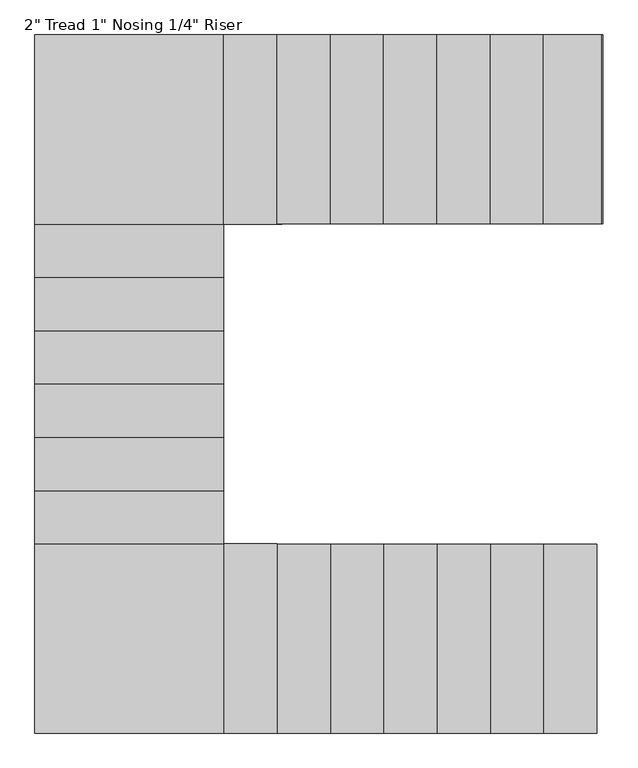
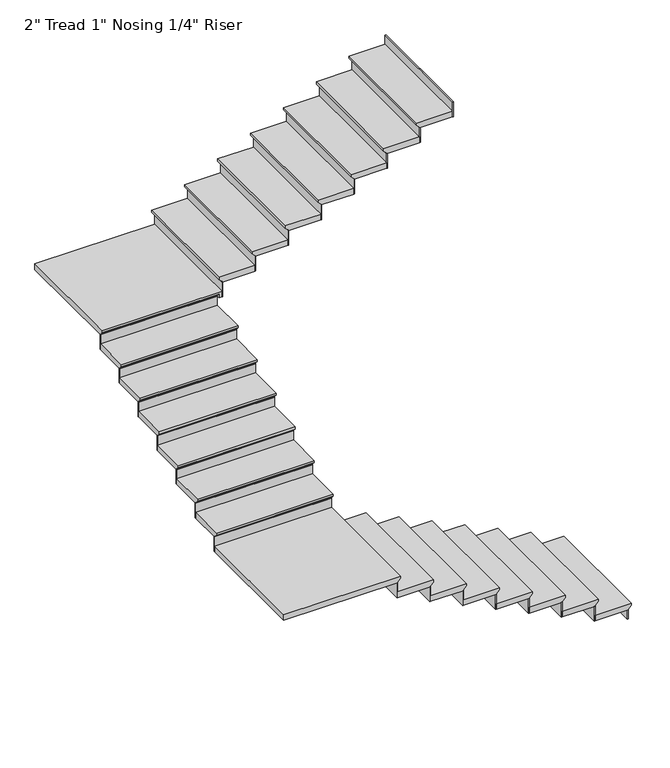
"""IFC4 building model written with IfcOpenShell, lengths in millimetres: stair flight geometry."""

from ifc_helpers import new_model, si_unit, origin, place, context, project, spatial, faceted_brep, source, transform, mapped, element, save


def stair_flight_9d362d5c(model_context):
    return source(origin(), model_context, "Body", "Brep", [
        faceted_brep([(-19769.8789184, -127.8399287, 3161.4717391), (-19769.8789184, -127.8399287, 3180.5217391), (-19769.8789184, -1118.4399287, 3180.5217391), (-19769.8789184, -1118.4399287, 3161.4717391), (-19795.2789184, -127.8399287, 3136.0717391), (-19795.2789184, -1118.4399287, 3136.0717391), (-20074.6789184, -127.8399287, 3180.5217391), (-20074.6789184, -1118.4399287, 3180.5217391), (-19795.2789184, -1118.4399287, 3129.7217391), (-20074.6789184, -1118.4399287, 3129.7217391), (-20074.6789184, -127.8399287, 3129.7217391), (-19795.2789184, -127.8399287, 3129.7217391)], [[[0, 1, 2, 3]], [[4, 0, 3, 5]], [[2, 1, 6, 7]], [[8, 9, 10, 11]], [[2, 7, 9, 8, 5, 3]], [[8, 11, 4, 5]], [[6, 1, 0, 4, 11, 10]], [[7, 6, 10, 9]]]),
        faceted_brep([(-19795.2789184, -127.8399287, 3129.7217391), (-19795.2789184, -127.8399287, 3048.0), (-19801.6289184, -127.8399287, 3048.0), (-19801.6289184, -127.8399287, 3129.7217391), (-19795.2789184, -1118.4399287, 3129.7217391), (-19801.6289184, -1118.4399287, 3129.7217391), (-19801.6289184, -1118.4399287, 3048.0), (-19795.2789184, -1118.4399287, 3048.0)], [[[0, 1, 2, 3]], [[4, 5, 6, 7]], [[1, 0, 4, 7]], [[2, 1, 7, 6]], [[3, 2, 6, 5]], [[0, 3, 5, 4]]]),
        faceted_brep([(-20074.6789184, -127.8399287, 3262.2434783), (-20074.6789184, -127.8399287, 3129.7217391), (-20081.0289184, -127.8399287, 3129.7217391), (-20081.0289184, -127.8399287, 3262.2434783), (-20074.6789184, -1118.4399287, 3262.2434783), (-20081.0289184, -1118.4399287, 3262.2434783), (-20081.0289184, -1118.4399287, 3129.7217391), (-20074.6789184, -1118.4399287, 3129.7217391)], [[[0, 1, 2, 3]], [[4, 5, 6, 7]], [[1, 0, 4, 7]], [[2, 1, 7, 6]], [[3, 2, 6, 5]], [[0, 3, 5, 4]]]),
        faceted_brep([(-20049.2789184, -1118.4399287, 3313.0434783), (-20049.2789184, -127.8399287, 3313.0434783), (-20354.0789184, -127.8399287, 3313.0434783), (-20354.0789184, -1118.4399287, 3313.0434783), (-20074.6789184, -1118.4399287, 3262.2434783), (-20354.0789184, -1118.4399287, 3262.2434783), (-20354.0789184, -127.8399287, 3262.2434783), (-20074.6789184, -127.8399287, 3262.2434783), (-20074.6789184, -1118.4399287, 3268.5934783), (-20049.2789184, -1118.4399287, 3293.9934783), (-20074.6789184, -127.8399287, 3268.5934783), (-20049.2789184, -127.8399287, 3293.9934783)], [[[0, 1, 2, 3]], [[4, 5, 6, 7]], [[0, 3, 5, 4, 8, 9]], [[4, 7, 10, 8]], [[2, 1, 11, 10, 7, 6]], [[3, 2, 6, 5]], [[11, 1, 0, 9]], [[10, 11, 9, 8]]]),
        faceted_brep([(-20354.0789184, -127.8399287, 3394.7652174), (-20354.0789184, -127.8399287, 3262.2434783), (-20360.4289184, -127.8399287, 3262.2434783), (-20360.4289184, -127.8399287, 3394.7652174), (-20354.0789184, -1118.4399287, 3394.7652174), (-20360.4289184, -1118.4399287, 3394.7652174), (-20360.4289184, -1118.4399287, 3262.2434783), (-20354.0789184, -1118.4399287, 3262.2434783)], [[[0, 1, 2, 3]], [[4, 5, 6, 7]], [[1, 0, 4, 7]], [[2, 1, 7, 6]], [[3, 2, 6, 5]], [[0, 3, 5, 4]]]),
        faceted_brep([(-20328.6789184, -1118.4399287, 3445.5652174), (-20328.6789184, -127.8399287, 3445.5652174), (-20633.4789184, -127.8399287, 3445.5652174), (-20633.4789184, -1118.4399287, 3445.5652174), (-20354.0789184, -1118.4399287, 3394.7652174), (-20633.4789184, -1118.4399287, 3394.7652174), (-20633.4789184, -127.8399287, 3394.7652174), (-20354.0789184, -127.8399287, 3394.7652174), (-20354.0789184, -1118.4399287, 3401.1152174), (-20328.6789184, -1118.4399287, 3426.5152174), (-20354.0789184, -127.8399287, 3401.1152174), (-20328.6789184, -127.8399287, 3426.5152174)], [[[0, 1, 2, 3]], [[4, 5, 6, 7]], [[0, 3, 5, 4, 8, 9]], [[4, 7, 10, 8]], [[2, 1, 11, 10, 7, 6]], [[3, 2, 6, 5]], [[11, 1, 0, 9]], [[10, 11, 9, 8]]]),
        faceted_brep([(-20633.4789184, -127.8399287, 3527.2869565), (-20633.4789184, -127.8399287, 3394.7652174), (-20639.8289184, -127.8399287, 3394.7652174), (-20639.8289184, -127.8399287, 3527.2869565), (-20633.4789184, -1118.4399287, 3527.2869565), (-20639.8289184, -1118.4399287, 3527.2869565), (-20639.8289184, -1118.4399287, 3394.7652174), (-20633.4789184, -1118.4399287, 3394.7652174)], [[[0, 1, 2, 3]], [[4, 5, 6, 7]], [[1, 0, 4, 7]], [[2, 1, 7, 6]], [[3, 2, 6, 5]], [[0, 3, 5, 4]]]),
        faceted_brep([(-20608.0789184, -1118.4399287, 3578.0869565), (-20608.0789184, -127.8399287, 3578.0869565), (-20912.8789184, -127.8399287, 3578.0869565), (-20912.8789184, -1118.4399287, 3578.0869565), (-20633.4789184, -1118.4399287, 3527.2869565), (-20912.8789184, -1118.4399287, 3527.2869565), (-20912.8789184, -127.8399287, 3527.2869565), (-20633.4789184, -127.8399287, 3527.2869565), (-20633.4789184, -1118.4399287, 3533.6369565), (-20608.0789184, -1118.4399287, 3559.0369565), (-20633.4789184, -127.8399287, 3533.6369565), (-20608.0789184, -127.8399287, 3559.0369565)], [[[0, 1, 2, 3]], [[4, 5, 6, 7]], [[0, 3, 5, 4, 8, 9]], [[4, 7, 10, 8]], [[2, 1, 11, 10, 7, 6]], [[3, 2, 6, 5]], [[11, 1, 0, 9]], [[10, 11, 9, 8]]]),
        faceted_brep([(-20912.8789184, -127.8399287, 3659.8086957), (-20912.8789184, -127.8399287, 3527.2869565), (-20919.2289184, -127.8399287, 3527.2869565), (-20919.2289184, -127.8399287, 3659.8086957), (-20912.8789184, -1118.4399287, 3659.8086957), (-20919.2289184, -1118.4399287, 3659.8086957), (-20919.2289184, -1118.4399287, 3527.2869565), (-20912.8789184, -1118.4399287, 3527.2869565)], [[[0, 1, 2, 3]], [[4, 5, 6, 7]], [[1, 0, 4, 7]], [[2, 1, 7, 6]], [[3, 2, 6, 5]], [[0, 3, 5, 4]]]),
        faceted_brep([(-20887.4789184, -1118.4399287, 3710.6086957), (-20887.4789184, -127.8399287, 3710.6086957), (-21192.2789184, -127.8399287, 3710.6086957), (-21192.2789184, -1118.4399287, 3710.6086957), (-20912.8789184, -1118.4399287, 3659.8086957), (-21192.2789184, -1118.4399287, 3659.8086957), (-21192.2789184, -127.8399287, 3659.8086957), (-20912.8789184, -127.8399287, 3659.8086957), (-20912.8789184, -1118.4399287, 3666.1586957), (-20887.4789184, -1118.4399287, 3691.5586957), (-20912.8789184, -127.8399287, 3666.1586957), (-20887.4789184, -127.8399287, 3691.5586957)], [[[0, 1, 2, 3]], [[4, 5, 6, 7]], [[0, 3, 5, 4, 8, 9]], [[4, 7, 10, 8]], [[2, 1, 11, 10, 7, 6]], [[3, 2, 6, 5]], [[11, 1, 0, 9]], [[10, 11, 9, 8]]]),
        faceted_brep([(-21192.2789184, -127.8399287, 3792.3304348), (-21192.2789184, -127.8399287, 3659.8086957), (-21198.6289184, -127.8399287, 3659.8086957), (-21198.6289184, -127.8399287, 3792.3304348), (-21192.2789184, -1118.4399287, 3792.3304348), (-21198.6289184, -1118.4399287, 3792.3304348), (-21198.6289184, -1118.4399287, 3659.8086957), (-21192.2789184, -1118.4399287, 3659.8086957)], [[[0, 1, 2, 3]], [[4, 5, 6, 7]], [[1, 0, 4, 7]], [[2, 1, 7, 6]], [[3, 2, 6, 5]], [[0, 3, 5, 4]]]),
        faceted_brep([(-21166.8789184, -1118.4399287, 3843.1304348), (-21166.8789184, -127.8399287, 3843.1304348), (-21471.6789184, -127.8399287, 3843.1304348), (-21471.6789184, -1118.4399287, 3843.1304348), (-21192.2789184, -1118.4399287, 3792.3304348), (-21471.6789184, -1118.4399287, 3792.3304348), (-21471.6789184, -127.8399287, 3792.3304348), (-21192.2789184, -127.8399287, 3792.3304348), (-21192.2789184, -1118.4399287, 3798.6804348), (-21166.8789184, -1118.4399287, 3824.0804348), (-21192.2789184, -127.8399287, 3798.6804348), (-21166.8789184, -127.8399287, 3824.0804348)], [[[0, 1, 2, 3]], [[4, 5, 6, 7]], [[0, 3, 5, 4, 8, 9]], [[4, 7, 10, 8]], [[2, 1, 11, 10, 7, 6]], [[3, 2, 6, 5]], [[11, 1, 0, 9]], [[10, 11, 9, 8]]]),
        faceted_brep([(-21471.6789184, -127.8399287, 3924.8521739), (-21471.6789184, -127.8399287, 3792.3304348), (-21478.0289184, -127.8399287, 3792.3304348), (-21478.0289184, -127.8399287, 3924.8521739), (-21471.6789184, -1118.4399287, 3924.8521739), (-21478.0289184, -1118.4399287, 3924.8521739), (-21478.0289184, -1118.4399287, 3792.3304348), (-21471.6789184, -1118.4399287, 3792.3304348)], [[[0, 1, 2, 3]], [[4, 5, 6, 7]], [[1, 0, 4, 7]], [[2, 1, 7, 6]], [[3, 2, 6, 5]], [[0, 3, 5, 4]]]),
        faceted_brep([(-21446.2789184, -1118.4399287, 3975.6521739), (-21446.2789184, -127.8399287, 3975.6521739), (-21751.0789184, -127.8399287, 3975.6521739), (-21751.0789184, -1118.4399287, 3975.6521739), (-21471.6789184, -1118.4399287, 3924.8521739), (-21751.0789184, -1118.4399287, 3924.8521739), (-21751.0789184, -127.8399287, 3924.8521739), (-21471.6789184, -127.8399287, 3924.8521739), (-21471.6789184, -1118.4399287, 3931.2021739), (-21446.2789184, -1118.4399287, 3956.6021739), (-21471.6789184, -127.8399287, 3931.2021739), (-21446.2789184, -127.8399287, 3956.6021739)], [[[0, 1, 2, 3]], [[4, 5, 6, 7]], [[0, 3, 5, 4, 8, 9]], [[4, 7, 10, 8]], [[2, 1, 11, 10, 7, 6]], [[3, 2, 6, 5]], [[11, 1, 0, 9]], [[10, 11, 9, 8]]]),
        faceted_brep([(-21751.0789184, -127.8399287, 4057.373913), (-21751.0789184, -127.8399287, 3924.8521739), (-21757.4289184, -127.8399287, 3924.8521739), (-21757.4289184, -127.8399287, 4057.373913), (-21751.0789184, -1118.4399287, 4057.373913), (-21757.4289184, -1118.4399287, 4057.373913), (-21757.4289184, -1118.4399287, 3924.8521739), (-21751.0789184, -1118.4399287, 3924.8521739)], [[[0, 1, 2, 3]], [[4, 5, 6, 7]], [[1, 0, 4, 7]], [[2, 1, 7, 6]], [[3, 2, 6, 5]], [[0, 3, 5, 4]]]),
        faceted_brep([(-22716.2789184, -102.4399287, 4108.173913), (-22716.2789184, -1118.4399287, 4108.173913), (-21725.6789184, -1118.4399287, 4108.173913), (-21725.6789184, -102.4399287, 4108.173913), (-22716.2789184, -1118.4399287, 4057.373913), (-22716.2789184, -102.4399287, 4057.373913), (-21725.6789184, -102.4399287, 4057.373913), (-21725.6789184, -127.8399287, 4057.373913), (-21751.0789184, -127.8399287, 4057.373913), (-21751.0789184, -1118.4399287, 4057.373913), (-21751.0789184, -127.8399287, 4063.723913), (-21751.0789184, -1118.4399287, 4063.723913), (-21725.6789184, -1118.4399287, 4089.123913), (-21725.6789184, -127.8399287, 4089.123913)], [[[0, 1, 2, 3]], [[4, 5, 6, 7, 8, 9]], [[1, 0, 5, 4]], [[9, 8, 10, 11]], [[3, 2, 12, 13, 7, 6]], [[0, 3, 6, 5]], [[12, 11, 10, 13]], [[2, 1, 4, 9, 11, 12]], [[8, 7, 13, 10]]]),
        faceted_brep([(-21725.6789184, -102.4399287, 4189.8956522), (-21725.6789184, -102.4399287, 4057.373913), (-21725.6789184, -96.0899287, 4057.373913), (-21725.6789184, -96.0899287, 4189.8956522), (-22716.2789184, -102.4399287, 4189.8956522), (-22716.2789184, -96.0899287, 4189.8956522), (-22716.2789184, -96.0899287, 4057.373913), (-22716.2789184, -102.4399287, 4057.373913)], [[[0, 1, 2, 3]], [[4, 5, 6, 7]], [[1, 0, 4, 7]], [[2, 1, 7, 6]], [[3, 2, 6, 5]], [[0, 3, 5, 4]]]),
        faceted_brep([(-22716.2789184, -127.8399287, 4240.6956522), (-21725.6789184, -127.8399287, 4240.6956522), (-21725.6789184, 176.9600713, 4240.6956522), (-22716.2789184, 176.9600713, 4240.6956522), (-22716.2789184, -102.4399287, 4189.8956522), (-22716.2789184, 176.9600713, 4189.8956522), (-21725.6789184, 176.9600713, 4189.8956522), (-21725.6789184, -102.4399287, 4189.8956522), (-22716.2789184, -102.4399287, 4196.2456522), (-22716.2789184, -127.8399287, 4221.6456522), (-21725.6789184, -102.4399287, 4196.2456522), (-21725.6789184, -127.8399287, 4221.6456522)], [[[0, 1, 2, 3]], [[4, 5, 6, 7]], [[0, 3, 5, 4, 8, 9]], [[4, 7, 10, 8]], [[2, 1, 11, 10, 7, 6]], [[3, 2, 6, 5]], [[11, 1, 0, 9]], [[10, 11, 9, 8]]]),
        faceted_brep([(-21725.6789184, 176.9600713, 4322.4173913), (-21725.6789184, 176.9600713, 4189.8956522), (-21725.6789184, 183.3100713, 4189.8956522), (-21725.6789184, 183.3100713, 4322.4173913), (-22716.2789184, 176.9600713, 4322.4173913), (-22716.2789184, 183.3100713, 4322.4173913), (-22716.2789184, 183.3100713, 4189.8956522), (-22716.2789184, 176.9600713, 4189.8956522)], [[[0, 1, 2, 3]], [[4, 5, 6, 7]], [[1, 0, 4, 7]], [[2, 1, 7, 6]], [[3, 2, 6, 5]], [[0, 3, 5, 4]]]),
        faceted_brep([(-22716.2789184, 151.5600713, 4373.2173913), (-21725.6789184, 151.5600713, 4373.2173913), (-21725.6789184, 456.3600713, 4373.2173913), (-22716.2789184, 456.3600713, 4373.2173913), (-22716.2789184, 176.9600713, 4322.4173913), (-22716.2789184, 456.3600713, 4322.4173913), (-21725.6789184, 456.3600713, 4322.4173913), (-21725.6789184, 176.9600713, 4322.4173913), (-22716.2789184, 176.9600713, 4328.7673913), (-22716.2789184, 151.5600713, 4354.1673913), (-21725.6789184, 176.9600713, 4328.7673913), (-21725.6789184, 151.5600713, 4354.1673913)], [[[0, 1, 2, 3]], [[4, 5, 6, 7]], [[0, 3, 5, 4, 8, 9]], [[4, 7, 10, 8]], [[2, 1, 11, 10, 7, 6]], [[3, 2, 6, 5]], [[11, 1, 0, 9]], [[10, 11, 9, 8]]]),
        faceted_brep([(-21725.6789184, 456.3600713, 4454.9391304), (-21725.6789184, 456.3600713, 4322.4173913), (-21725.6789184, 462.7100713, 4322.4173913), (-21725.6789184, 462.7100713, 4454.9391304), (-22716.2789184, 456.3600713, 4454.9391304), (-22716.2789184, 462.7100713, 4454.9391304), (-22716.2789184, 462.7100713, 4322.4173913), (-22716.2789184, 456.3600713, 4322.4173913)], [[[0, 1, 2, 3]], [[4, 5, 6, 7]], [[1, 0, 4, 7]], [[2, 1, 7, 6]], [[3, 2, 6, 5]], [[0, 3, 5, 4]]]),
        faceted_brep([(-22716.2789184, 430.9600713, 4505.7391304), (-21725.6789184, 430.9600713, 4505.7391304), (-21725.6789184, 735.7600713, 4505.7391304), (-22716.2789184, 735.7600713, 4505.7391304), (-22716.2789184, 456.3600713, 4454.9391304), (-22716.2789184, 735.7600713, 4454.9391304), (-21725.6789184, 735.7600713, 4454.9391304), (-21725.6789184, 456.3600713, 4454.9391304), (-22716.2789184, 456.3600713, 4461.2891304), (-22716.2789184, 430.9600713, 4486.6891304), (-21725.6789184, 456.3600713, 4461.2891304), (-21725.6789184, 430.9600713, 4486.6891304)], [[[0, 1, 2, 3]], [[4, 5, 6, 7]], [[0, 3, 5, 4, 8, 9]], [[4, 7, 10, 8]], [[2, 1, 11, 10, 7, 6]], [[3, 2, 6, 5]], [[11, 1, 0, 9]], [[10, 11, 9, 8]]]),
        faceted_brep([(-21725.6789184, 735.7600713, 4587.4608696), (-21725.6789184, 735.7600713, 4454.9391304), (-21725.6789184, 742.1100713, 4454.9391304), (-21725.6789184, 742.1100713, 4587.4608696), (-22716.2789184, 735.7600713, 4587.4608696), (-22716.2789184, 742.1100713, 4587.4608696), (-22716.2789184, 742.1100713, 4454.9391304), (-22716.2789184, 735.7600713, 4454.9391304)], [[[0, 1, 2, 3]], [[4, 5, 6, 7]], [[1, 0, 4, 7]], [[2, 1, 7, 6]], [[3, 2, 6, 5]], [[0, 3, 5, 4]]]),
        faceted_brep([(-22716.2789184, 710.3600713, 4638.2608696), (-21725.6789184, 710.3600713, 4638.2608696), (-21725.6789184, 1015.1600713, 4638.2608696), (-22716.2789184, 1015.1600713, 4638.2608696), (-22716.2789184, 735.7600713, 4587.4608696), (-22716.2789184, 1015.1600713, 4587.4608696), (-21725.6789184, 1015.1600713, 4587.4608696), (-21725.6789184, 735.7600713, 4587.4608696), (-22716.2789184, 735.7600713, 4593.8108696), (-22716.2789184, 710.3600713, 4619.2108696), (-21725.6789184, 735.7600713, 4593.8108696), (-21725.6789184, 710.3600713, 4619.2108696)], [[[0, 1, 2, 3]], [[4, 5, 6, 7]], [[0, 3, 5, 4, 8, 9]], [[4, 7, 10, 8]], [[2, 1, 11, 10, 7, 6]], [[3, 2, 6, 5]], [[11, 1, 0, 9]], [[10, 11, 9, 8]]]),
        faceted_brep([(-21725.6789184, 1015.1600713, 4719.9826087), (-21725.6789184, 1015.1600713, 4587.4608696), (-21725.6789184, 1021.5100713, 4587.4608696), (-21725.6789184, 1021.5100713, 4719.9826087), (-22716.2789184, 1015.1600713, 4719.9826087), (-22716.2789184, 1021.5100713, 4719.9826087), (-22716.2789184, 1021.5100713, 4587.4608696), (-22716.2789184, 1015.1600713, 4587.4608696)], [[[0, 1, 2, 3]], [[4, 5, 6, 7]], [[1, 0, 4, 7]], [[2, 1, 7, 6]], [[3, 2, 6, 5]], [[0, 3, 5, 4]]]),
        faceted_brep([(-22716.2789184, 989.7600713, 4770.7826087), (-21725.6789184, 989.7600713, 4770.7826087), (-21725.6789184, 1294.5600713, 4770.7826087), (-22716.2789184, 1294.5600713, 4770.7826087), (-22716.2789184, 1015.1600713, 4719.9826087), (-22716.2789184, 1294.5600713, 4719.9826087), (-21725.6789184, 1294.5600713, 4719.9826087), (-21725.6789184, 1015.1600713, 4719.9826087), (-22716.2789184, 1015.1600713, 4726.3326087), (-22716.2789184, 989.7600713, 4751.7326087), (-21725.6789184, 1015.1600713, 4726.3326087), (-21725.6789184, 989.7600713, 4751.7326087)], [[[0, 1, 2, 3]], [[4, 5, 6, 7]], [[0, 3, 5, 4, 8, 9]], [[4, 7, 10, 8]], [[2, 1, 11, 10, 7, 6]], [[3, 2, 6, 5]], [[11, 1, 0, 9]], [[10, 11, 9, 8]]]),
        faceted_brep([(-21725.6789184, 1294.5600713, 4852.5043478), (-21725.6789184, 1294.5600713, 4719.9826087), (-21725.6789184, 1300.9100713, 4719.9826087), (-21725.6789184, 1300.9100713, 4852.5043478), (-22716.2789184, 1294.5600713, 4852.5043478), (-22716.2789184, 1300.9100713, 4852.5043478), (-22716.2789184, 1300.9100713, 4719.9826087), (-22716.2789184, 1294.5600713, 4719.9826087)], [[[0, 1, 2, 3]], [[4, 5, 6, 7]], [[1, 0, 4, 7]], [[2, 1, 7, 6]], [[3, 2, 6, 5]], [[0, 3, 5, 4]]]),
        faceted_brep([(-22716.2789184, 1269.1600713, 4903.3043478), (-21725.6789184, 1269.1600713, 4903.3043478), (-21725.6789184, 1573.9600713, 4903.3043478), (-22716.2789184, 1573.9600713, 4903.3043478), (-22716.2789184, 1294.5600713, 4852.5043478), (-22716.2789184, 1573.9600713, 4852.5043478), (-21725.6789184, 1573.9600713, 4852.5043478), (-21725.6789184, 1294.5600713, 4852.5043478), (-22716.2789184, 1294.5600713, 4858.8543478), (-22716.2789184, 1269.1600713, 4884.2543478), (-21725.6789184, 1294.5600713, 4858.8543478), (-21725.6789184, 1269.1600713, 4884.2543478)], [[[0, 1, 2, 3]], [[4, 5, 6, 7]], [[0, 3, 5, 4, 8, 9]], [[4, 7, 10, 8]], [[2, 1, 11, 10, 7, 6]], [[3, 2, 6, 5]], [[11, 1, 0, 9]], [[10, 11, 9, 8]]]),
        faceted_brep([(-21725.6789184, 1573.9600713, 4985.026087), (-21725.6789184, 1573.9600713, 4852.5043478), (-21725.6789184, 1580.3100713, 4852.5043478), (-21725.6789184, 1580.3100713, 4985.026087), (-22716.2789184, 1573.9600713, 4985.026087), (-22716.2789184, 1580.3100713, 4985.026087), (-22716.2789184, 1580.3100713, 4852.5043478), (-22716.2789184, 1573.9600713, 4852.5043478)], [[[0, 1, 2, 3]], [[4, 5, 6, 7]], [[1, 0, 4, 7]], [[2, 1, 7, 6]], [[3, 2, 6, 5]], [[0, 3, 5, 4]]]),
        faceted_brep([(-21700.2789184, 2539.1600713, 5035.826087), (-22716.2789184, 2539.1600713, 5035.826087), (-22716.2789184, 1548.5600713, 5035.826087), (-21700.2789184, 1548.5600713, 5035.826087), (-22716.2789184, 2539.1600713, 4985.026087), (-21700.2789184, 2539.1600713, 4985.026087), (-21700.2789184, 1548.5600713, 4985.026087), (-21725.6789184, 1548.5600713, 4985.026087), (-21725.6789184, 1573.9600713, 4985.026087), (-22716.2789184, 1573.9600713, 4985.026087), (-21725.6789184, 1573.9600713, 4991.376087), (-22716.2789184, 1573.9600713, 4991.376087), (-22716.2789184, 1548.5600713, 5016.776087), (-21725.6789184, 1548.5600713, 5016.776087)], [[[0, 1, 2, 3]], [[4, 5, 6, 7, 8, 9]], [[1, 0, 5, 4]], [[9, 8, 10, 11]], [[3, 2, 12, 13, 7, 6]], [[0, 3, 6, 5]], [[12, 11, 10, 13]], [[2, 1, 4, 9, 11, 12]], [[8, 7, 13, 10]]]),
        faceted_brep([(-21700.2789184, 1548.5600713, 5117.5478261), (-21700.2789184, 1548.5600713, 4985.026087), (-21693.9289184, 1548.5600713, 4985.026087), (-21693.9289184, 1548.5600713, 5117.5478261), (-21700.2789184, 2539.1600713, 5117.5478261), (-21693.9289184, 2539.1600713, 5117.5478261), (-21693.9289184, 2539.1600713, 4985.026087), (-21700.2789184, 2539.1600713, 4985.026087)], [[[0, 1, 2, 3]], [[4, 5, 6, 7]], [[1, 0, 4, 7]], [[2, 1, 7, 6]], [[3, 2, 6, 5]], [[0, 3, 5, 4]]]),
        faceted_brep([(-21725.6789184, 2539.1600713, 5168.3478261), (-21725.6789184, 1548.5600713, 5168.3478261), (-21420.8789184, 1548.5600713, 5168.3478261), (-21420.8789184, 2539.1600713, 5168.3478261), (-21700.2789184, 2539.1600713, 5117.5478261), (-21420.8789184, 2539.1600713, 5117.5478261), (-21420.8789184, 1548.5600713, 5117.5478261), (-21700.2789184, 1548.5600713, 5117.5478261), (-21700.2789184, 2539.1600713, 5123.8978261), (-21725.6789184, 2539.1600713, 5149.2978261), (-21700.2789184, 1548.5600713, 5123.8978261), (-21725.6789184, 1548.5600713, 5149.2978261)], [[[0, 1, 2, 3]], [[4, 5, 6, 7]], [[0, 3, 5, 4, 8, 9]], [[4, 7, 10, 8]], [[2, 1, 11, 10, 7, 6]], [[3, 2, 6, 5]], [[11, 1, 0, 9]], [[10, 11, 9, 8]]]),
        faceted_brep([(-21420.8789184, 1548.5600713, 5250.0695652), (-21420.8789184, 1548.5600713, 5117.5478261), (-21414.5289184, 1548.5600713, 5117.5478261), (-21414.5289184, 1548.5600713, 5250.0695652), (-21420.8789184, 2539.1600713, 5250.0695652), (-21414.5289184, 2539.1600713, 5250.0695652), (-21414.5289184, 2539.1600713, 5117.5478261), (-21420.8789184, 2539.1600713, 5117.5478261)], [[[0, 1, 2, 3]], [[4, 5, 6, 7]], [[1, 0, 4, 7]], [[2, 1, 7, 6]], [[3, 2, 6, 5]], [[0, 3, 5, 4]]]),
        faceted_brep([(-21446.2789184, 2539.1600713, 5300.8695652), (-21446.2789184, 1548.5600713, 5300.8695652), (-21141.4789184, 1548.5600713, 5300.8695652), (-21141.4789184, 2539.1600713, 5300.8695652), (-21420.8789184, 2539.1600713, 5250.0695652), (-21141.4789184, 2539.1600713, 5250.0695652), (-21141.4789184, 1548.5600713, 5250.0695652), (-21420.8789184, 1548.5600713, 5250.0695652), (-21420.8789184, 2539.1600713, 5256.4195652), (-21446.2789184, 2539.1600713, 5281.8195652), (-21420.8789184, 1548.5600713, 5256.4195652), (-21446.2789184, 1548.5600713, 5281.8195652)], [[[0, 1, 2, 3]], [[4, 5, 6, 7]], [[0, 3, 5, 4, 8, 9]], [[4, 7, 10, 8]], [[2, 1, 11, 10, 7, 6]], [[3, 2, 6, 5]], [[11, 1, 0, 9]], [[10, 11, 9, 8]]]),
        faceted_brep([(-21141.4789184, 1548.5600713, 5382.5913043), (-21141.4789184, 1548.5600713, 5250.0695652), (-21135.1289184, 1548.5600713, 5250.0695652), (-21135.1289184, 1548.5600713, 5382.5913043), (-21141.4789184, 2539.1600713, 5382.5913043), (-21135.1289184, 2539.1600713, 5382.5913043), (-21135.1289184, 2539.1600713, 5250.0695652), (-21141.4789184, 2539.1600713, 5250.0695652)], [[[0, 1, 2, 3]], [[4, 5, 6, 7]], [[1, 0, 4, 7]], [[2, 1, 7, 6]], [[3, 2, 6, 5]], [[0, 3, 5, 4]]]),
        faceted_brep([(-21166.8789184, 2539.1600713, 5433.3913043), (-21166.8789184, 1548.5600713, 5433.3913043), (-20862.0789184, 1548.5600713, 5433.3913043), (-20862.0789184, 2539.1600713, 5433.3913043), (-21141.4789184, 2539.1600713, 5382.5913043), (-20862.0789184, 2539.1600713, 5382.5913043), (-20862.0789184, 1548.5600713, 5382.5913043), (-21141.4789184, 1548.5600713, 5382.5913043), (-21141.4789184, 2539.1600713, 5388.9413043), (-21166.8789184, 2539.1600713, 5414.3413043), (-21141.4789184, 1548.5600713, 5388.9413043), (-21166.8789184, 1548.5600713, 5414.3413043)], [[[0, 1, 2, 3]], [[4, 5, 6, 7]], [[0, 3, 5, 4, 8, 9]], [[4, 7, 10, 8]], [[2, 1, 11, 10, 7, 6]], [[3, 2, 6, 5]], [[11, 1, 0, 9]], [[10, 11, 9, 8]]]),
        faceted_brep([(-20862.0789184, 1548.5600713, 5515.1130435), (-20862.0789184, 1548.5600713, 5382.5913043), (-20855.7289184, 1548.5600713, 5382.5913043), (-20855.7289184, 1548.5600713, 5515.1130435), (-20862.0789184, 2539.1600713, 5515.1130435), (-20855.7289184, 2539.1600713, 5515.1130435), (-20855.7289184, 2539.1600713, 5382.5913043), (-20862.0789184, 2539.1600713, 5382.5913043)], [[[0, 1, 2, 3]], [[4, 5, 6, 7]], [[1, 0, 4, 7]], [[2, 1, 7, 6]], [[3, 2, 6, 5]], [[0, 3, 5, 4]]]),
        faceted_brep([(-20887.4789184, 2539.1600713, 5565.9130435), (-20887.4789184, 1548.5600713, 5565.9130435), (-20582.6789184, 1548.5600713, 5565.9130435), (-20582.6789184, 2539.1600713, 5565.9130435), (-20862.0789184, 2539.1600713, 5515.1130435), (-20582.6789184, 2539.1600713, 5515.1130435), (-20582.6789184, 1548.5600713, 5515.1130435), (-20862.0789184, 1548.5600713, 5515.1130435), (-20862.0789184, 2539.1600713, 5521.4630435), (-20887.4789184, 2539.1600713, 5546.8630435), (-20862.0789184, 1548.5600713, 5521.4630435), (-20887.4789184, 1548.5600713, 5546.8630435)], [[[0, 1, 2, 3]], [[4, 5, 6, 7]], [[0, 3, 5, 4, 8, 9]], [[4, 7, 10, 8]], [[2, 1, 11, 10, 7, 6]], [[3, 2, 6, 5]], [[11, 1, 0, 9]], [[10, 11, 9, 8]]]),
        faceted_brep([(-20582.6789184, 1548.5600713, 5647.6347826), (-20582.6789184, 1548.5600713, 5515.1130435), (-20576.3289184, 1548.5600713, 5515.1130435), (-20576.3289184, 1548.5600713, 5647.6347826), (-20582.6789184, 2539.1600713, 5647.6347826), (-20576.3289184, 2539.1600713, 5647.6347826), (-20576.3289184, 2539.1600713, 5515.1130435), (-20582.6789184, 2539.1600713, 5515.1130435)], [[[0, 1, 2, 3]], [[4, 5, 6, 7]], [[1, 0, 4, 7]], [[2, 1, 7, 6]], [[3, 2, 6, 5]], [[0, 3, 5, 4]]]),
        faceted_brep([(-20608.0789184, 2539.1600713, 5698.4347826), (-20608.0789184, 1548.5600713, 5698.4347826), (-20303.2789184, 1548.5600713, 5698.4347826), (-20303.2789184, 2539.1600713, 5698.4347826), (-20582.6789184, 2539.1600713, 5647.6347826), (-20303.2789184, 2539.1600713, 5647.6347826), (-20303.2789184, 1548.5600713, 5647.6347826), (-20582.6789184, 1548.5600713, 5647.6347826), (-20582.6789184, 2539.1600713, 5653.9847826), (-20608.0789184, 2539.1600713, 5679.3847826), (-20582.6789184, 1548.5600713, 5653.9847826), (-20608.0789184, 1548.5600713, 5679.3847826)], [[[0, 1, 2, 3]], [[4, 5, 6, 7]], [[0, 3, 5, 4, 8, 9]], [[4, 7, 10, 8]], [[2, 1, 11, 10, 7, 6]], [[3, 2, 6, 5]], [[11, 1, 0, 9]], [[10, 11, 9, 8]]]),
        faceted_brep([(-20303.2789184, 1548.5600713, 5780.1565217), (-20303.2789184, 1548.5600713, 5647.6347826), (-20296.9289184, 1548.5600713, 5647.6347826), (-20296.9289184, 1548.5600713, 5780.1565217), (-20303.2789184, 2539.1600713, 5780.1565217), (-20296.9289184, 2539.1600713, 5780.1565217), (-20296.9289184, 2539.1600713, 5647.6347826), (-20303.2789184, 2539.1600713, 5647.6347826)], [[[0, 1, 2, 3]], [[4, 5, 6, 7]], [[1, 0, 4, 7]], [[2, 1, 7, 6]], [[3, 2, 6, 5]], [[0, 3, 5, 4]]]),
        faceted_brep([(-20328.6789184, 2539.1600713, 5830.9565217), (-20328.6789184, 1548.5600713, 5830.9565217), (-20023.8789184, 1548.5600713, 5830.9565217), (-20023.8789184, 2539.1600713, 5830.9565217), (-20303.2789184, 2539.1600713, 5780.1565217), (-20023.8789184, 2539.1600713, 5780.1565217), (-20023.8789184, 1548.5600713, 5780.1565217), (-20303.2789184, 1548.5600713, 5780.1565217), (-20303.2789184, 2539.1600713, 5786.5065217), (-20328.6789184, 2539.1600713, 5811.9065217), (-20303.2789184, 1548.5600713, 5786.5065217), (-20328.6789184, 1548.5600713, 5811.9065217)], [[[0, 1, 2, 3]], [[4, 5, 6, 7]], [[0, 3, 5, 4, 8, 9]], [[4, 7, 10, 8]], [[2, 1, 11, 10, 7, 6]], [[3, 2, 6, 5]], [[11, 1, 0, 9]], [[10, 11, 9, 8]]]),
        faceted_brep([(-20023.8789184, 1548.5600713, 5912.6782609), (-20023.8789184, 1548.5600713, 5780.1565217), (-20017.5289184, 1548.5600713, 5780.1565217), (-20017.5289184, 1548.5600713, 5912.6782609), (-20023.8789184, 2539.1600713, 5912.6782609), (-20017.5289184, 2539.1600713, 5912.6782609), (-20017.5289184, 2539.1600713, 5780.1565217), (-20023.8789184, 2539.1600713, 5780.1565217)], [[[0, 1, 2, 3]], [[4, 5, 6, 7]], [[1, 0, 4, 7]], [[2, 1, 7, 6]], [[3, 2, 6, 5]], [[0, 3, 5, 4]]]),
        faceted_brep([(-19744.4789184, 1548.5600713, 6045.2), (-19744.4789184, 1548.5600713, 5912.6782609), (-19738.1289184, 1548.5600713, 5912.6782609), (-19738.1289184, 1548.5600713, 6045.2), (-19744.4789184, 2539.1600713, 6045.2), (-19738.1289184, 2539.1600713, 6045.2), (-19738.1289184, 2539.1600713, 5912.6782609), (-19744.4789184, 2539.1600713, 5912.6782609)], [[[0, 1, 2, 3]], [[4, 5, 6, 7]], [[1, 0, 4, 7]], [[2, 1, 7, 6]], [[3, 2, 6, 5]], [[0, 3, 5, 4]]]),
        faceted_brep([(-20049.2789184, 2539.1600713, 5963.4782609), (-20049.2789184, 1548.5600713, 5963.4782609), (-19744.4789184, 1548.5600713, 5963.4782609), (-19744.4789184, 2539.1600713, 5963.4782609), (-20023.8789184, 2539.1600713, 5912.6782609), (-19744.4789184, 2539.1600713, 5912.6782609), (-19744.4789184, 1548.5600713, 5912.6782609), (-20023.8789184, 1548.5600713, 5912.6782609), (-20023.8789184, 2539.1600713, 5919.0282609), (-20049.2789184, 2539.1600713, 5944.4282609), (-20023.8789184, 1548.5600713, 5919.0282609), (-20049.2789184, 1548.5600713, 5944.4282609)], [[[0, 1, 2, 3]], [[4, 5, 6, 7]], [[0, 3, 5, 4, 8, 9]], [[4, 7, 10, 8]], [[2, 1, 11, 10, 7, 6]], [[3, 2, 6, 5]], [[11, 1, 0, 9]], [[10, 11, 9, 8]]]),
    ])


if __name__ == "__main__":
    model = new_model("IFC4")
    model_context = context("Model", 3, world=origin())
    ifc_project = project(units=[si_unit("LENGTHUNIT", "METRE", prefix="MILLI")], contexts=[model_context])
    site = spatial("IfcSite", under=ifc_project)
    building = spatial("IfcBuilding", under=site)
    placement = place(None, origin())
    stair_flight_shape = stair_flight_9d362d5c(model_context)
    element("IfcStairFlight", 1, ObjectType="2\" Tread 1\" Nosing 1/4\" Riser", at=placement, inside=building, context=model_context, shape_type="MappedRepresentation", body=[
        mapped(stair_flight_shape, transform((0.0, 0.0, 0.0), x_axis=(1.0, 0.0, 0.0), y_axis=(0.0, 1.0, 0.0), z_axis=(0.0, 0.0, 1.0))),
    ])
    save(model, "model.ifc")
